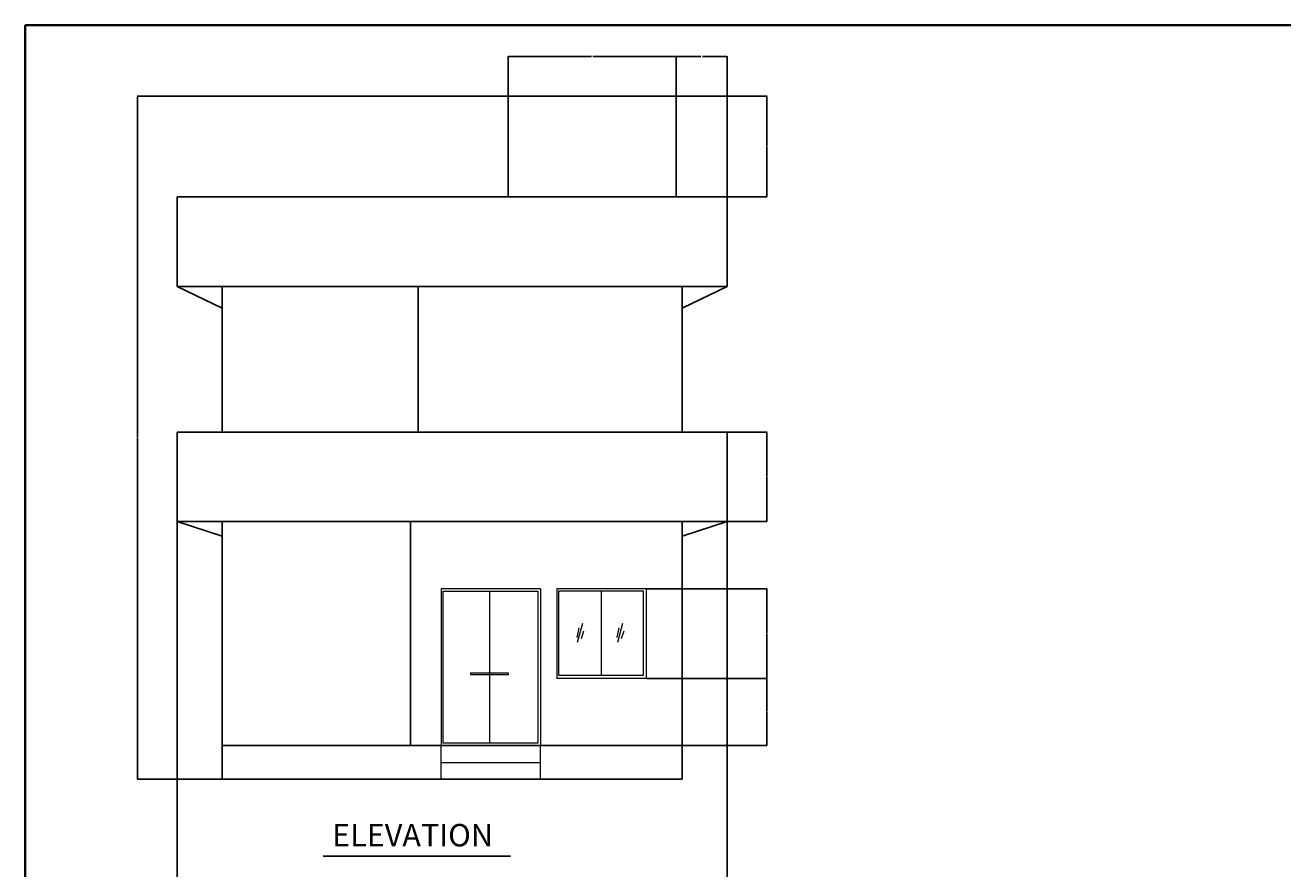
# Model space of a CAD drawing. Units: inches. Extents: x 1911 to 3278, y 2022 to 3108.
# Tile 10 of 13: x 1911 to 2585, y 2656 to 3108. Entities that reach past the tile are written whole.
import ezdxf

# ---------------------------------------------------------------- set-up
doc = ezdxf.new("R2010")
doc.units = ezdxf.units.IN
for name, color, linetype, lineweight in [('A-ANNO-DIMS', 2, 'Continuous', 18), ('A-ANNO-TITL', 7, 'Continuous', 25), ('A-ANNO-TTLB', 7, 'Continuous', 35), ('A-DOOR', 4, 'Continuous', 18), ('A-ELEV', 7, 'Continuous', 25), ('A-FLOR-STRS', 7, 'Continuous', 18), ('A-GLAZ', 4, 'Continuous', 18)]:
    doc.layers.add(name, color=color, linetype=linetype, lineweight=lineweight)
doc.styles.get("Standard").update_dxf_attribs({"font": 'arial.ttf'})
doc.dimstyles.get("Standard").update_dxf_attribs({"dimtxt": 0.18, "dimasz": 0.18, "dimexe": 0.18, "dimexo": 0.0625, "dimgap": 0.09, "dimtad": 0, "dimtih": 1, "dimtoh": 1, "dimdec": 4, "dimzin": 0, "dimdsep": 46, "dimtxsty": 'Standard', "dimcen": 0.09, "dimadec": 0, "dimazin": 0, "dimtfac": 1, "dimtdec": 4, "dimtofl": 0, "dimtmove": 0, "dimatfit": 3, "dimfxl": 1, "dimtolj": 1, "dimtzin": 0, "dimarcsym": 0})

# ---------------------------------------------------------------- blocks, each defined once
blk = doc.blocks.new('*D89')
at = {"layer": 'A-ANNO-DIMS', "color": 0, "lineweight": -2, "transparency": 16777216}
for p, q in [((1992.83, 2841.96), (1992.83, 2641.37)), ((2287.33, 2841.96), (2287.33, 2641.37)), ((1993.01, 2641.55), (2139.69, 2641.55)), ((2287.15, 2641.55), (2140.48, 2641.55))]:
    blk.add_line(p, q, dxfattribs=at)
at = {"layer": 'A-ANNO-DIMS', "color": 0, "transparency": 16777216}
for points in [[(1993.01, 2641.58), (1993.01, 2641.52), (1992.83, 2641.55)], [(2287.15, 2641.58), (2287.15, 2641.52), (2287.33, 2641.55)]]:
    blk.add_solid(points, dxfattribs=at)
at = {"layer": 'Defpoints', "color": 0, "transparency": 16777216}
for p in [(1992.83, 2842.03), (2287.33, 2842.03), (2287.33, 2641.55)]:
    blk.add_point(p, dxfattribs=at)
at = {"layer": 'A-ANNO-DIMS', "color": 0, "transparency": 16777216, "insert": (2140.08, 2641.55), "char_height": 0.18, "attachment_point": 5}
blk.add_mtext('\\A1;294.5', dxfattribs=at)
blk = doc.blocks.new('*D90')
at = {"layer": 'A-ANNO-DIMS', "color": 0, "lineweight": -2, "transparency": 16777216}
for p, q in [((2169.94, 3070), (1971.45, 3070)), ((1971.63, 3069.82), (1971.63, 2887.2)), ((1971.63, 2704.21), (1971.63, 2886.83)), ((2016.77, 2704.03), (1971.45, 2704.03))]:
    blk.add_line(p, q, dxfattribs=at)
at = {"layer": 'A-ANNO-DIMS', "color": 0, "transparency": 16777216}
for points in [[(1971.6, 3069.82), (1971.66, 3069.82), (1971.63, 3070)], [(1971.6, 2704.21), (1971.66, 2704.21), (1971.63, 2704.03)]]:
    blk.add_solid(points, dxfattribs=at)
at = {"layer": 'Defpoints', "color": 0, "transparency": 16777216}
for p in [(1971.63, 3070), (2170, 3070), (2016.83, 2704.03)]:
    blk.add_point(p, dxfattribs=at)
at = {"layer": 'A-ANNO-DIMS', "color": 0, "transparency": 16777216, "insert": (1971.63, 2887.01), "char_height": 0.18, "attachment_point": 5}
blk.add_mtext('\\A1;366', dxfattribs=at)
blk = doc.blocks.new('*D91')
at = {"layer": 'A-ANNO-DIMS', "color": 0, "lineweight": -2, "transparency": 16777216}
for p, q in [((2244.1, 2758.03), (2308.71, 2758.03)), ((2308.53, 2757.85), (2308.53, 2740.21)), ((2308.53, 2722.21), (2308.53, 2739.85)), ((2263.4, 2722.03), (2308.71, 2722.03))]:
    blk.add_line(p, q, dxfattribs=at)
at = {"layer": 'A-ANNO-DIMS', "color": 0, "transparency": 16777216}
for points in [[(2308.5, 2757.85), (2308.56, 2757.85), (2308.53, 2758.03)], [(2308.5, 2722.21), (2308.56, 2722.21), (2308.53, 2722.03)]]:
    blk.add_solid(points, dxfattribs=at)
at = {"layer": 'Defpoints', "color": 0, "transparency": 16777216}
for p in [(2244.04, 2758.03), (2308.53, 2758.03), (2263.33, 2722.03)]:
    blk.add_point(p, dxfattribs=at)
at = {"layer": 'A-ANNO-DIMS', "color": 0, "transparency": 16777216, "insert": (2308.53, 2740.03), "char_height": 0.18, "attachment_point": 5}
blk.add_mtext('\\A1;36', dxfattribs=at)
blk = doc.blocks.new('*D92')
at = {"layer": 'A-ANNO-DIMS', "color": 0, "lineweight": -2, "transparency": 16777216}
for p, q in [((2244.1, 2806.03), (2308.71, 2806.03)), ((2308.53, 2805.85), (2308.53, 2782.21)), ((2308.53, 2758.21), (2308.53, 2781.85)), ((2244.1, 2758.03), (2308.71, 2758.03))]:
    blk.add_line(p, q, dxfattribs=at)
at = {"layer": 'A-ANNO-DIMS', "color": 0, "transparency": 16777216}
for points in [[(2308.5, 2805.85), (2308.56, 2805.85), (2308.53, 2806.03)], [(2308.5, 2758.21), (2308.56, 2758.21), (2308.53, 2758.03)]]:
    blk.add_solid(points, dxfattribs=at)
at = {"layer": 'Defpoints', "color": 0, "transparency": 16777216}
for p in [(2244.04, 2806.03), (2308.53, 2806.03), (2244.04, 2758.03)]:
    blk.add_point(p, dxfattribs=at)
at = {"layer": 'A-ANNO-DIMS', "color": 0, "transparency": 16777216, "insert": (2308.53, 2782.03), "char_height": 0.18, "attachment_point": 5}
blk.add_mtext('\\A1;48', dxfattribs=at)
blk = doc.blocks.new('*D93')
at = {"layer": 'A-ANNO-DIMS', "color": 0, "lineweight": -2, "transparency": 16777216}
for p, q in [((2287.4, 2890.03), (2308.71, 2890.03)), ((2308.53, 2889.85), (2308.53, 2866.21)), ((2308.53, 2842.21), (2308.53, 2865.85)), ((2287.4, 2842.03), (2308.71, 2842.03))]:
    blk.add_line(p, q, dxfattribs=at)
at = {"layer": 'A-ANNO-DIMS', "color": 0, "transparency": 16777216}
for points in [[(2308.5, 2889.85), (2308.56, 2889.85), (2308.53, 2890.03)], [(2308.5, 2842.21), (2308.56, 2842.21), (2308.53, 2842.03)]]:
    blk.add_solid(points, dxfattribs=at)
at = {"layer": 'Defpoints', "color": 0, "transparency": 16777216}
for p in [(2287.33, 2890.03), (2308.53, 2890.03), (2287.33, 2842.03)]:
    blk.add_point(p, dxfattribs=at)
at = {"layer": 'A-ANNO-DIMS', "color": 0, "transparency": 16777216, "insert": (2308.53, 2866.03), "char_height": 0.18, "attachment_point": 5}
blk.add_mtext('\\A1;48', dxfattribs=at)
blk = doc.blocks.new('*D94')
at = {"layer": 'A-ANNO-DIMS', "color": 0, "lineweight": -2, "transparency": 16777216}
for p, q in [((2260.15, 3070), (2308.71, 3070)), ((2308.53, 3069.82), (2308.53, 3043.2)), ((2308.53, 3016.21), (2308.53, 3042.83)), ((2260.15, 3016.03), (2308.71, 3016.03))]:
    blk.add_line(p, q, dxfattribs=at)
at = {"layer": 'A-ANNO-DIMS', "color": 0, "transparency": 16777216}
for points in [[(2308.5, 3069.82), (2308.56, 3069.82), (2308.53, 3070)], [(2308.5, 3016.21), (2308.56, 3016.21), (2308.53, 3016.03)]]:
    blk.add_solid(points, dxfattribs=at)
at = {"layer": 'Defpoints', "color": 0, "transparency": 16777216}
for p in [(2260.08, 3070), (2308.53, 3070), (2260.08, 3016.03)]:
    blk.add_point(p, dxfattribs=at)
at = {"layer": 'A-ANNO-DIMS', "color": 0, "transparency": 16777216, "insert": (2308.53, 3043.01), "char_height": 0.18, "attachment_point": 5}
blk.add_mtext('\\A1;53.97', dxfattribs=at)
blk = doc.blocks.new('*D95')
at = {"layer": 'A-ANNO-DIMS', "color": 0, "lineweight": -2, "transparency": 16777216}
for p, q in [((2170, 3070.06), (2170, 3091.38)), ((2170.18, 3091.2), (2214.65, 3091.2)), ((2259.9, 3091.2), (2215.44, 3091.2)), ((2260.08, 3070.06), (2260.08, 3091.38))]:
    blk.add_line(p, q, dxfattribs=at)
at = {"layer": 'A-ANNO-DIMS', "color": 0, "transparency": 16777216}
for points in [[(2170.18, 3091.23), (2170.18, 3091.17), (2170, 3091.2)], [(2259.9, 3091.23), (2259.9, 3091.17), (2260.08, 3091.2)]]:
    blk.add_solid(points, dxfattribs=at)
at = {"layer": 'Defpoints', "color": 0, "transparency": 16777216}
for p in [(2260.08, 3091.2), (2170, 3070), (2260.08, 3070)]:
    blk.add_point(p, dxfattribs=at)
at = {"layer": 'A-ANNO-DIMS', "color": 0, "transparency": 16777216, "insert": (2215.04, 3091.2), "char_height": 0.18, "attachment_point": 5}
blk.add_mtext('\\A1;90.08', dxfattribs=at)
blk = doc.blocks.new('*D96')
at = {"layer": 'A-ANNO-DIMS', "color": 0, "lineweight": -2, "transparency": 16777216}
for p, q in [((2260.08, 3070.06), (2260.08, 3091.38)), ((2260.26, 3091.2), (2273.31, 3091.2)), ((2287.15, 3091.2), (2274.11, 3091.2)), ((2287.33, 3016.09), (2287.33, 3091.38))]:
    blk.add_line(p, q, dxfattribs=at)
at = {"layer": 'A-ANNO-DIMS', "color": 0, "transparency": 16777216}
for points in [[(2260.26, 3091.23), (2260.26, 3091.17), (2260.08, 3091.2)], [(2287.15, 3091.23), (2287.15, 3091.17), (2287.33, 3091.2)]]:
    blk.add_solid(points, dxfattribs=at)
at = {"layer": 'Defpoints', "color": 0, "transparency": 16777216}
for p in [(2287.33, 3091.2), (2260.08, 3070), (2287.33, 3016.03)]:
    blk.add_point(p, dxfattribs=at)
at = {"layer": 'A-ANNO-DIMS', "color": 0, "transparency": 16777216, "insert": (2273.71, 3091.2), "char_height": 0.18, "attachment_point": 5}
blk.add_mtext('\\A1;27.25', dxfattribs=at)

msp = doc.modelspace()

# ---------------------------------------------------------------- linework, layer by layer
at = {"layer": 'A-ANNO-TITL'}
msp.add_line((2070.9135, 2662.7501), (2171.3665, 2662.7501), dxfattribs=at)
at = {"layer": 'A-ANNO-TTLB'}
msp.add_lwpolyline([(1911.3875, 3108.0628), (3278.3142, 3108.0628), (3278.3142, 2021.7237), (1911.3875, 2021.7237)], close=True, dxfattribs=at)
at = {"layer": 'A-DOOR'}
for p, q in [((2134.1034, 2806.0271), (2134.1034, 2722.0271)), ((2187.3146, 2806.0271), (2134.1034, 2806.0271)), ((2160, 2804.821), (2160, 2723.2543)), ((2187.3146, 2806.0271), (2187.3146, 2722.0271))]:
    msp.add_line(p, q, dxfattribs=at)
for points in [[(2135.2296, 2804.821), (2186.0259, 2804.821), (2186.0259, 2723.2543), (2135.2296, 2723.2543)], [(2150, 2761.0764), (2160, 2761.0764), (2160, 2760), (2150, 2760)], [(2160, 2761.0764), (2170, 2761.0764), (2170, 2760), (2160, 2760)]]:
    msp.add_lwpolyline(points, close=True, dxfattribs=at)
at = {"layer": 'A-ELEV'}
for p, q in [((2260.0844, 3070), (2170, 3070)), ((2170, 3070), (2170, 3016.0271)), ((2260.0844, 3016.0271), (2260.0844, 3070)), ((2287.3344, 3016.0271), (1992.8344, 3016.0271)), ((1992.8344, 2968.0271), (1992.8344, 3016.0271)), ((2263.3344, 3016.0271), (2256.8344, 3016.0271)), ((2287.3344, 2968.0271), (2287.3344, 3016.0271)), ((2287.3344, 2968.0271), (1992.8344, 2968.0271)), ((1992.8344, 2968.0271), (2016.8344, 2956.3859)), ((2016.8344, 2968.0271), (2016.8344, 2890.0271)), ((2121.8344, 2968.0271), (2121.8344, 2890.0271)), ((2263.3344, 2890.0271), (2263.3344, 2968.0271)), ((2287.3344, 2968.0271), (2263.3344, 2956.4386)), ((2287.3344, 2890.0271), (1992.8344, 2890.0271)), ((1992.8344, 2842.0271), (1992.8344, 2890.0271)), ((2287.3344, 2842.0271), (2287.3344, 2890.0271)), ((2287.3344, 2842.0271), (1992.8344, 2842.0271)), ((1992.8344, 2842.0271), (2016.8344, 2834.2605)), ((2016.8344, 2842.0271), (2016.8344, 2704.0271)), ((2016.8344, 2842.0271), (2016.8344, 2830.0271)), ((2117.8344, 2842.0271), (2117.8344, 2722.0271)), ((2263.3344, 2842.0271), (2263.3344, 2704.0271)), ((2287.3344, 2842.0271), (2263.3344, 2834.2956)), ((2263.3344, 2722.0271), (2016.8344, 2722.0271)), ((2263.3344, 2704.0271), (2016.8344, 2704.0271))]:
    msp.add_line(p, q, dxfattribs=at)
at = {"layer": 'A-FLOR-STRS'}
msp.add_line((2134.1034, 2713.0271), (2187.1717, 2713.0271), dxfattribs=at)
msp.add_lwpolyline([(2134.1034, 2722.0271), (2187.1717, 2722.0271), (2187.1717, 2704.0271), (2134.1034, 2704.0271)], close=True, dxfattribs=at)
at = {"layer": 'A-GLAZ'}
for p, q in [((2196.0406, 2806.0271), (2196.0406, 2758.0271)), ((2244.0406, 2806.0271), (2196.0406, 2806.0271)), ((2219.7837, 2804.9144), (2219.7837, 2759.5609)), ((2244.0406, 2806.0271), (2244.0406, 2758.0271)), ((2207.8318, 2785.0997), (2206.7932, 2779.8846)), ((2209.8312, 2787.3568), (2207.0561, 2777.2472)), ((2210.4308, 2783.2679), (2209.1185, 2779.2943)), ((2229.3626, 2785.0997), (2228.324, 2779.8846)), ((2231.362, 2787.3568), (2228.5869, 2777.2472)), ((2231.9616, 2783.2679), (2230.6494, 2779.2943)), ((2244.0406, 2758.0271), (2196.0406, 2758.0271))]:
    msp.add_line(p, q, dxfattribs=at)
msp.add_lwpolyline([(2197.2284, 2804.9144), (2242.339, 2804.9144), (2242.339, 2759.5609), (2197.2284, 2759.5609)], close=True, dxfattribs=at)

# ---------------------------------------------------------------- texts
at = {"layer": 'A-ANNO-TITL', "insert": (2075.8001, 2680), "char_height": 12, "attachment_point": 1}
msp.add_mtext_dynamic_manual_height_columns('ELEVATION', width=210, gutter_width=12.5, heights=[0], dxfattribs=at)

# ---------------------------------------------------------------- dimensions: what is measured, and where the dimension line sits
at = {"layer": 'A-ANNO-DIMS'}
for base, p1, p2, override, picture, middle in [((2260.0844, 3091.2), (2170, 3070), (2260.0844, 3070), {"dimdec": 2, "dimlfac": 1, "dimrnd": 0, "dimzin": 0, "dimdsep": 46, "dimlunit": 2}, '*D95', (2215.0422, 3091.2)), ((2287.3344, 3091.2), (2260.0844, 3070), (2287.3344, 3016.0271), {"dimdec": 2, "dimlfac": 1, "dimrnd": 0, "dimzin": 0, "dimdsep": 46, "dimlunit": 2}, '*D96', (2273.7094, 3091.2)), ((2287.3344, 2641.5501), (1992.8344, 2842.0271), (2287.3344, 2842.0271), {"dimdec": 1, "dimlfac": 1, "dimrnd": 0, "dimzin": 0, "dimdsep": 46, "dimlunit": 2}, '*D89', (2140.0844, 2641.5501))]:
    dim = msp.add_linear_dim(base=base, p1=p1, p2=p2, dimstyle='Standard', override=override, dxfattribs=at)
    dim.commit()
    dim.dimension.update_dxf_attribs({"geometry": picture, "text_midpoint": middle})
for base, p1, p2, override, picture, middle in [((1971.6344, 3070), (2016.8344, 2704.0271), (2170, 3070), {"dimdec": 0, "dimlfac": 1, "dimrnd": 0, "dimzin": 0, "dimdsep": 46, "dimlunit": 2}, '*D90', (1971.6344, 2887.0135)), ((2308.5344, 3070), (2260.0844, 3016.0271), (2260.0844, 3070), {"dimdec": 2, "dimlfac": 1, "dimrnd": 0, "dimzin": 0, "dimdsep": 46, "dimlunit": 2}, '*D94', (2308.5344, 3043.0135)), ((2308.5344, 2890.0271), (2287.3344, 2842.0271), (2287.3344, 2890.0271), {"dimdec": 0, "dimlfac": 1, "dimrnd": 0, "dimzin": 0, "dimdsep": 46, "dimlunit": 2}, '*D93', (2308.5344, 2866.0271)), ((2308.5344, 2806.0271), (2244.0406, 2758.0271), (2244.0406, 2806.0271), {"dimdec": 0, "dimlfac": 1, "dimrnd": 0, "dimzin": 0, "dimdsep": 46, "dimlunit": 2}, '*D92', (2308.5344, 2782.0271)), ((2308.5344, 2758.0271), (2263.3344, 2722.0271), (2244.0406, 2758.0271), {"dimdec": 0, "dimlfac": 1, "dimrnd": 0, "dimzin": 0, "dimdsep": 46, "dimlunit": 2}, '*D91', (2308.5344, 2740.0271))]:
    dim = msp.add_linear_dim(base=base, p1=p1, p2=p2, angle=90, dimstyle='Standard', override=override, dxfattribs=at)
    dim.commit()
    dim.dimension.update_dxf_attribs({"geometry": picture, "text_midpoint": middle})

doc.saveas('drawing.dxf')
